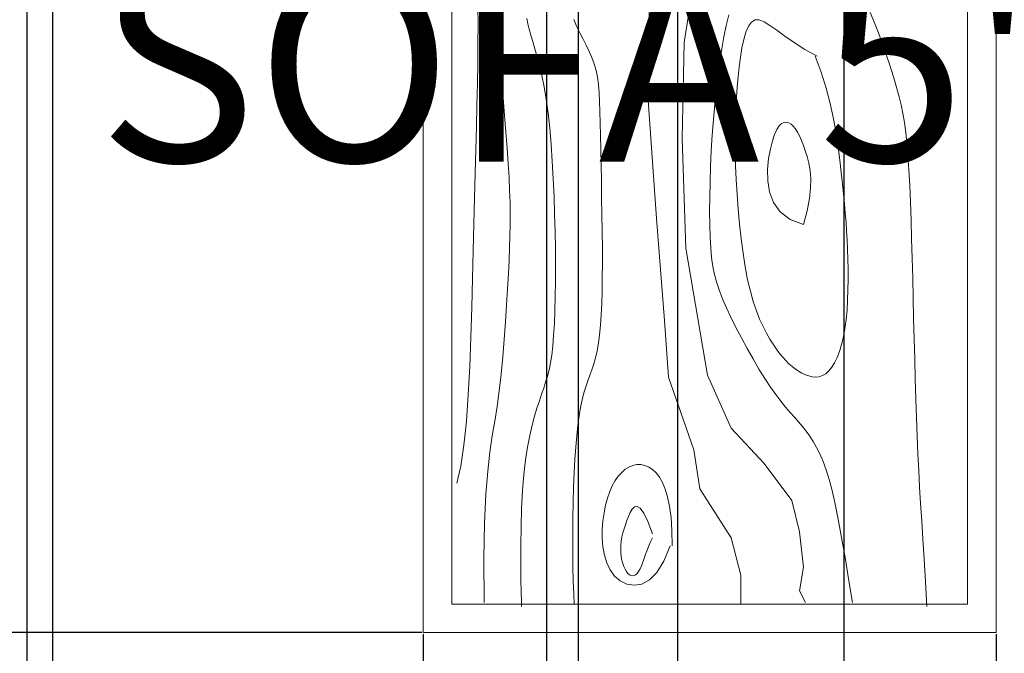
# Model space of a CAD drawing. Units: inches. Extents: x -26 to 385, y 12 to 697.
# Tile 6 of 13: x 223 to 264, y 165 to 191. Entities that reach past the tile are written whole.
import ezdxf

# ---------------------------------------------------------------- set-up
doc = ezdxf.new("R2010")
doc.units = ezdxf.units.IN
doc.header["$MEASUREMENT"] = 0
doc.layers.add('A-ANNO-DIMS', color=4, linetype='Continuous', lineweight=18)
doc.layers.add('Furniture', color=210, linetype='Continuous', lineweight=15)
doc.styles.get("Standard").update_dxf_attribs({"font": 'italic8.shx'})
doc.dimstyles.get("Standard").update_dxf_attribs({"dimtxt": 8, "dimasz": 0.18, "dimexe": 0.18, "dimexo": 0.0625, "dimgap": 0.09, "dimtad": 0, "dimtih": 1, "dimtoh": 1, "dimdec": 4, "dimzin": 0, "dimdsep": 46, "dimlunit": 3, "dimtxsty": 'Standard', "dimcen": 0.09, "dimclrd": 2, "dimclre": 3, "dimclrt": 6, "dimadec": 0, "dimazin": 0, "dimtfac": 1, "dimtdec": 4, "dimtofl": 0, "dimtmove": 0, "dimatfit": 3, "dimfxl": 1, "dimtolj": 1, "dimtzin": 0, "dimarcsym": 0})

# ---------------------------------------------------------------- blocks, each defined once
blk = doc.blocks.new('*D11')
at = {"layer": 'A-ANNO-DIMS', "color": 3, "lineweight": -2, "transparency": 16777216}
for p, q in [((285.56, 224.402), (274.992, 224.402)), ((285.56, 154.738), (274.992, 154.738))]:
    blk.add_line(p, q, dxfattribs=at)
at = {"layer": 'A-ANNO-DIMS', "color": 2, "lineweight": -2, "transparency": 16777216}
for p, q in [((275.172, 224.222), (275.172, 195.755)), ((275.172, 154.918), (275.172, 183.384))]:
    blk.add_line(p, q, dxfattribs=at)
at = {"layer": 'A-ANNO-DIMS', "color": 2, "transparency": 16777216}
for points in [[(275.142, 224.222), (275.202, 224.222), (275.172, 224.402)], [(275.142, 154.918), (275.202, 154.918), (275.172, 154.738)]]:
    blk.add_solid(points, dxfattribs=at)
at = {"layer": 'Defpoints', "color": 0, "transparency": 16777216}
for p in [(285.622, 224.402), (275.172, 154.738), (285.622, 154.738)]:
    blk.add_point(p, dxfattribs=at)
at = {"layer": 'A-ANNO-DIMS', "color": 6, "transparency": 16777216, "insert": (275.172, 189.57), "char_height": 8, "attachment_point": 5}
blk.add_mtext('\\A1;SOFA 5\'-9 1/2" TYP.', dxfattribs=at)
blk = doc.blocks.new('*D28')
at = {"layer": 'A-ANNO-DIMS', "color": 3, "lineweight": -2, "transparency": 16777216}
for p, q in [((141.692, 194.903), (355.559, 194.903)), ((141.692, 158.903), (355.559, 158.903))]:
    blk.add_line(p, q, dxfattribs=at)
at = {"layer": 'A-ANNO-DIMS', "color": 2, "lineweight": -2, "transparency": 16777216}
for p, q in [((355.379, 194.723), (355.379, 181.755)), ((355.379, 159.083), (355.379, 172.052))]:
    blk.add_line(p, q, dxfattribs=at)
at = {"layer": 'A-ANNO-DIMS', "color": 2, "transparency": 16777216}
for points in [[(355.349, 194.723), (355.409, 194.723), (355.379, 194.903)], [(355.349, 159.083), (355.409, 159.083), (355.379, 158.903)]]:
    blk.add_solid(points, dxfattribs=at)
at = {"layer": 'Defpoints', "color": 0, "transparency": 16777216}
for p in [(141.629, 194.903), (355.379, 194.903), (141.629, 158.903)]:
    blk.add_point(p, dxfattribs=at)
at = {"layer": 'A-ANNO-DIMS', "color": 6, "transparency": 16777216, "insert": (355.379, 176.903), "char_height": 8, "attachment_point": 5}
blk.add_mtext('\\A1;3\'-0"', dxfattribs=at)
blk = doc.blocks.new('*D31')
at = {"layer": 'A-ANNO-DIMS', "color": 3, "lineweight": -2, "transparency": 16777216}
for p, q in [((239.888, 166.079), (239.888, 23.949)), ((263.51, 166.079), (263.51, 23.949))]:
    blk.add_line(p, q, dxfattribs=at)
at = {"layer": 'A-ANNO-DIMS', "color": 2, "lineweight": -2, "transparency": 16777216}
for p, q in [((240.068, 24.129), (263.33, 24.129)), ((263.51, 24.129), (263.69, 24.129))]:
    blk.add_line(p, q, dxfattribs=at)
at = {"layer": 'A-ANNO-DIMS', "color": 2, "transparency": 16777216}
for points in [[(240.068, 24.159), (240.068, 24.099), (239.888, 24.129)], [(263.33, 24.159), (263.33, 24.099), (263.51, 24.129)]]:
    blk.add_solid(points, dxfattribs=at)
at = {"layer": 'Defpoints', "color": 0, "transparency": 16777216}
for p in [(239.888, 166.141), (263.51, 166.141), (263.51, 24.129)]:
    blk.add_point(p, dxfattribs=at)
at = {"layer": 'A-ANNO-DIMS', "color": 6, "transparency": 16777216, "insert": (296.732, 24.129), "char_height": 8, "attachment_point": 5}
blk.add_mtext('\\A1;1\'-11 1/2"', dxfattribs=at)
blk = doc.blocks.new('*D32')
at = {"layer": 'A-ANNO-DIMS', "color": 3, "lineweight": -2, "transparency": 16777216}
for p, q in [((239.825, 213.385), (-5.301, 213.385)), ((239.825, 166.141), (-5.301, 166.141))]:
    blk.add_line(p, q, dxfattribs=at)
at = {"layer": 'A-ANNO-DIMS', "color": 2, "lineweight": -2, "transparency": 16777216}
for p, q in [((-5.121, 213.205), (-5.121, 194.615)), ((-5.121, 166.321), (-5.121, 184.911))]:
    blk.add_line(p, q, dxfattribs=at)
at = {"layer": 'A-ANNO-DIMS', "color": 2, "transparency": 16777216}
for points in [[(-5.151, 213.205), (-5.091, 213.205), (-5.121, 213.385)], [(-5.151, 166.321), (-5.091, 166.321), (-5.121, 166.141)]]:
    blk.add_solid(points, dxfattribs=at)
at = {"layer": 'Defpoints', "color": 0, "transparency": 16777216}
for p in [(-5.121, 213.385), (239.888, 213.385), (239.888, 166.141)]:
    blk.add_point(p, dxfattribs=at)
at = {"layer": 'A-ANNO-DIMS', "color": 6, "transparency": 16777216, "insert": (-5.121, 189.763), "char_height": 8, "attachment_point": 5}
blk.add_mtext('\\A1;3\'-11"', dxfattribs=at)
blk = doc.blocks.new('*D35')
at = {"layer": 'A-ANNO-DIMS', "color": 3, "lineweight": -2, "transparency": 16777216}
for p, q in [((193.598, 147.942), (193.598, 684.809)), ((244.986, 147.942), (244.986, 684.809))]:
    blk.add_line(p, q, dxfattribs=at)
at = {"layer": 'A-ANNO-DIMS', "color": 2, "lineweight": -2, "transparency": 16777216}
for p, q in [((193.778, 684.629), (244.806, 684.629)), ((244.986, 684.629), (245.166, 684.629))]:
    blk.add_line(p, q, dxfattribs=at)
at = {"layer": 'A-ANNO-DIMS', "color": 2, "transparency": 16777216}
for points in [[(193.778, 684.659), (193.778, 684.599), (193.598, 684.629)], [(244.806, 684.659), (244.806, 684.599), (244.986, 684.629)]]:
    blk.add_solid(points, dxfattribs=at)
at = {"layer": 'Defpoints', "color": 0, "transparency": 16777216}
for p in [(244.986, 684.629), (193.598, 147.879), (244.986, 147.879)]:
    blk.add_point(p, dxfattribs=at)
at = {"layer": 'A-ANNO-DIMS', "color": 6, "transparency": 16777216, "insert": (278.398, 684.629), "char_height": 8, "attachment_point": 5}
blk.add_mtext('\\A1;4\'-3 1/2"', dxfattribs=at)
blk = doc.blocks.new('*D36')
at = {"layer": 'A-ANNO-DIMS', "color": 3, "lineweight": -2, "transparency": 16777216}
for p, q in [((146.129, 147.942), (146.129, 684.809)), ((193.598, 147.942), (193.598, 684.809))]:
    blk.add_line(p, q, dxfattribs=at)
at = {"layer": 'A-ANNO-DIMS', "color": 2, "lineweight": -2, "transparency": 16777216}
for p, q in [((146.309, 684.629), (193.418, 684.629)), ((193.598, 684.629), (193.778, 684.629))]:
    blk.add_line(p, q, dxfattribs=at)
at = {"layer": 'A-ANNO-DIMS', "color": 2, "transparency": 16777216}
for points in [[(146.309, 684.659), (146.309, 684.599), (146.129, 684.629)], [(193.418, 684.659), (193.418, 684.599), (193.598, 684.629)]]:
    blk.add_solid(points, dxfattribs=at)
at = {"layer": 'Defpoints', "color": 0, "transparency": 16777216}
for p in [(193.598, 684.629), (146.129, 147.879), (193.598, 147.879)]:
    blk.add_point(p, dxfattribs=at)
at = {"layer": 'A-ANNO-DIMS', "color": 6, "transparency": 16777216, "insert": (228.344, 684.629), "char_height": 8, "attachment_point": 5}
blk.add_mtext('\\A1;3\'-11 1/2"', dxfattribs=at)
blk = doc.blocks.new('*D37')
at = {"layer": 'A-ANNO-DIMS', "color": 3, "lineweight": -2, "transparency": 16777216}
for p, q in [((223.549, 597.317), (223.549, 23.949)), ((257.22, 597.317), (257.22, 23.949))]:
    blk.add_line(p, q, dxfattribs=at)
at = {"layer": 'A-ANNO-DIMS', "color": 2, "lineweight": -2, "transparency": 16777216}
for p, q in [((223.729, 24.129), (257.04, 24.129)), ((257.22, 24.129), (257.4, 24.129))]:
    blk.add_line(p, q, dxfattribs=at)
at = {"layer": 'A-ANNO-DIMS', "color": 2, "transparency": 16777216}
for points in [[(223.729, 24.159), (223.729, 24.099), (223.549, 24.129)], [(257.04, 24.159), (257.04, 24.099), (257.22, 24.129)]]:
    blk.add_solid(points, dxfattribs=at)
at = {"layer": 'Defpoints', "color": 0, "transparency": 16777216}
for p in [(223.549, 597.379), (257.22, 597.379), (257.22, 24.129)]:
    blk.add_point(p, dxfattribs=at)
at = {"layer": 'A-ANNO-DIMS', "color": 6, "transparency": 16777216, "insert": (290.633, 24.129), "char_height": 8, "attachment_point": 5}
blk.add_mtext('\\A1;2\'-9 1/2"', dxfattribs=at)
blk = doc.blocks.new('*D39')
at = {"layer": 'A-ANNO-DIMS', "color": 3, "lineweight": -2, "transparency": 16777216}
for p, q in [((183.359, 597.317), (183.359, 23.949)), ((213.359, 597.317), (213.359, 23.949))]:
    blk.add_line(p, q, dxfattribs=at)
at = {"layer": 'A-ANNO-DIMS', "color": 2, "lineweight": -2, "transparency": 16777216}
for p, q in [((183.539, 24.129), (213.179, 24.129)), ((213.359, 24.129), (213.539, 24.129))]:
    blk.add_line(p, q, dxfattribs=at)
at = {"layer": 'A-ANNO-DIMS', "color": 2, "transparency": 16777216}
for points in [[(183.539, 24.159), (183.539, 24.099), (183.359, 24.129)], [(213.179, 24.159), (213.179, 24.099), (213.359, 24.129)]]:
    blk.add_solid(points, dxfattribs=at)
at = {"layer": 'Defpoints', "color": 0, "transparency": 16777216}
for p in [(183.359, 597.379), (213.359, 597.379), (213.359, 24.129)]:
    blk.add_point(p, dxfattribs=at)
at = {"layer": 'A-ANNO-DIMS', "color": 6, "transparency": 16777216, "insert": (231.533, 24.129), "char_height": 8, "attachment_point": 5}
blk.add_mtext('\\A1;2\'-6"', dxfattribs=at)
blk = doc.blocks.new('*D42')
at = {"layer": 'A-ANNO-DIMS', "color": 3, "lineweight": -2, "transparency": 16777216}
for p, q in [((250.371, 518.992), (250.371, 23.949)), ((274.129, 518.992), (274.129, 23.949))]:
    blk.add_line(p, q, dxfattribs=at)
at = {"layer": 'A-ANNO-DIMS', "color": 2, "lineweight": -2, "transparency": 16777216}
for p, q in [((250.551, 24.129), (273.949, 24.129)), ((274.129, 24.129), (274.309, 24.129))]:
    blk.add_line(p, q, dxfattribs=at)
at = {"layer": 'A-ANNO-DIMS', "color": 2, "transparency": 16777216}
for points in [[(250.551, 24.159), (250.551, 24.099), (250.371, 24.129)], [(273.949, 24.159), (273.949, 24.099), (274.129, 24.129)]]:
    blk.add_solid(points, dxfattribs=at)
at = {"layer": 'Defpoints', "color": 0, "transparency": 16777216}
for p in [(250.371, 519.055), (274.129, 519.055), (274.129, 24.129)]:
    blk.add_point(p, dxfattribs=at)
at = {"layer": 'A-ANNO-DIMS', "color": 6, "transparency": 16777216, "insert": (292.304, 24.129), "char_height": 8, "attachment_point": 5}
blk.add_mtext('\\A1;2\'-0"', dxfattribs=at)
blk = doc.blocks.new('*D46')
at = {"layer": 'A-ANNO-DIMS', "color": 3, "lineweight": -2, "transparency": 16777216}
for p, q in [((224.595, 477.317), (224.595, 23.949)), ((284.629, 477.317), (284.629, 23.949))]:
    blk.add_line(p, q, dxfattribs=at)
at = {"layer": 'A-ANNO-DIMS', "color": 2, "lineweight": -2, "transparency": 16777216}
for p, q in [((224.775, 24.129), (236.617, 24.129)), ((284.449, 24.129), (272.607, 24.129))]:
    blk.add_line(p, q, dxfattribs=at)
at = {"layer": 'A-ANNO-DIMS', "color": 2, "transparency": 16777216}
for points in [[(224.775, 24.159), (224.775, 24.099), (224.595, 24.129)], [(284.449, 24.159), (284.449, 24.099), (284.629, 24.129)]]:
    blk.add_solid(points, dxfattribs=at)
at = {"layer": 'Defpoints', "color": 0, "transparency": 16777216}
for p in [(224.595, 477.379), (284.629, 477.379), (284.629, 24.129)]:
    blk.add_point(p, dxfattribs=at)
at = {"layer": 'A-ANNO-DIMS', "color": 6, "transparency": 16777216, "insert": (254.612, 24.129), "char_height": 8, "attachment_point": 5}
blk.add_mtext('\\A1;5\'-0"', dxfattribs=at)
blk = doc.blocks.new('*D50')
at = {"layer": 'A-ANNO-DIMS', "color": 3, "lineweight": -2, "transparency": 16777216}
for p, q in [((246.278, 401.871), (246.278, 23.949)), ((284.629, 398.317), (284.629, 23.949))]:
    blk.add_line(p, q, dxfattribs=at)
at = {"layer": 'A-ANNO-DIMS', "color": 2, "lineweight": -2, "transparency": 16777216}
for p, q in [((246.458, 24.129), (284.449, 24.129)), ((284.629, 24.129), (284.809, 24.129))]:
    blk.add_line(p, q, dxfattribs=at)
at = {"layer": 'A-ANNO-DIMS', "color": 2, "transparency": 16777216}
for points in [[(246.458, 24.159), (246.458, 24.099), (246.278, 24.129)], [(284.449, 24.159), (284.449, 24.099), (284.629, 24.129)]]:
    blk.add_solid(points, dxfattribs=at)
at = {"layer": 'Defpoints', "color": 0, "transparency": 16777216}
for p in [(246.278, 401.934), (284.629, 398.379), (284.629, 24.129)]:
    blk.add_point(p, dxfattribs=at)
at = {"layer": 'A-ANNO-DIMS', "color": 6, "transparency": 16777216, "insert": (318.042, 24.129), "char_height": 8, "attachment_point": 5}
blk.add_mtext('\\A1;3\'-2 1/2"', dxfattribs=at)

msp = doc.modelspace()

# ---------------------------------------------------------------- linework, layer by layer
at = {"layer": 'Furniture'}
for p, q in [((239.88756, 166.14113), (239.88756, 213.38513)), ((263.50956, 213.38513), (263.50956, 166.14113)), ((241.06866, 167.32223), (241.06866, 212.20403)), ((262.32846, 212.20403), (262.32846, 167.32223)), ((249.26214, 193.39853), (249.10065, 188.87448)), ((251.1193, 193.47931), (250.63482, 190.49021)), ((242.14138, 191.96625), (242.1424, 191.22463)), ((242.85064, 191.86926), (242.91269, 191.14289)), ((252.47852, 191.62122), (252.37572, 191.18868)), ((258.31298, 191.71684), (258.48609, 191.29892)), ((242.1424, 191.22463), (242.13822, 190.4475)), ((244.16233, 191.47311), (244.20257, 191.25411)), ((244.20257, 191.25411), (244.25591, 191.02879)), ((246.08743, 191.4343), (246.20915, 191.15418)), ((252.37572, 191.18868), (252.27939, 190.72079)), ((253.28986, 191.15523), (253.41478, 191.3285)), ((253.41478, 191.3285), (253.56186, 191.41926)), ((253.56186, 191.41926), (253.73411, 191.41965)), ((253.73411, 191.41965), (253.93688, 191.3391)), ((253.93688, 191.3391), (254.17608, 191.19133)), ((254.17608, 191.19133), (254.45763, 190.99008)), ((258.48609, 191.29892), (258.64973, 190.88226)), ((242.91269, 191.14289), (242.97743, 190.40942)), ((244.25591, 191.02879), (244.32351, 190.7868)), ((244.32351, 190.7868), (244.4031, 190.52177)), ((246.20915, 191.15418), (246.33876, 190.88541)), ((246.33876, 190.88541), (246.47137, 190.62486)), ((253.09673, 190.60971), (253.18466, 190.91158)), ((253.18466, 190.91158), (253.28986, 191.15523)), ((254.45763, 190.99008), (254.78743, 190.74906)), ((258.64973, 190.88226), (258.8036, 190.47001)), ((242.13822, 190.4475), (242.12931, 189.63661)), ((242.97743, 190.40942), (243.04343, 189.66972)), ((244.4031, 190.52177), (244.49152, 190.22834)), ((246.47137, 190.62486), (246.60208, 190.36935)), ((250.63482, 190.49021), (250.55408, 186.53167)), ((252.27939, 190.72079), (252.18968, 190.22008)), ((253.02362, 190.26176), (253.09673, 190.60971)), ((254.78743, 190.74906), (255.17141, 190.48201)), ((255.17141, 190.48201), (255.61547, 190.20265)), ((258.8036, 190.47001), (258.94738, 190.06535)), ((244.49152, 190.22834), (244.58562, 189.90114)), ((246.60208, 190.36935), (246.72601, 190.11573)), ((246.72601, 190.11573), (246.83827, 189.86085)), ((252.18968, 190.22008), (252.10675, 189.68908)), ((252.96289, 189.87989), (253.02362, 190.26176)), ((255.61547, 190.20265), (256.12553, 189.9247)), ((258.94738, 190.06535), (259.08074, 189.67141)), ((242.12931, 189.63661), (242.11614, 188.79369)), ((243.04343, 189.66972), (243.10927, 188.93002)), ((244.58562, 189.90114), (244.68224, 189.53481)), ((246.83827, 189.86085), (246.93397, 189.60156)), ((246.93397, 189.60156), (247.00954, 189.33403)), ((252.10675, 189.68908), (252.03076, 189.1303)), ((252.91209, 189.47625), (252.96289, 189.87989)), ((256.04479, 189.9247), (256.29361, 189.26091)), ((259.08074, 189.67141), (259.20339, 189.29135)), ((244.68224, 189.53481), (244.77823, 189.12399)), ((247.00954, 189.33403), (247.06666, 189.05183)), ((252.86879, 189.06298), (252.91209, 189.47625)), ((256.29361, 189.26091), (256.49867, 188.60572)), ((259.20339, 189.29135), (259.31499, 188.92834)), ((242.11614, 188.79369), (242.09919, 187.91978)), ((243.10927, 188.93002), (243.17354, 188.19789)), ((244.77823, 189.12399), (244.87044, 188.66331)), ((247.06666, 189.05183), (247.10832, 188.74786)), ((247.10832, 188.74786), (247.13752, 188.41501)), ((249.10065, 188.87448), (249.50438, 183.21942)), ((252.03076, 189.1303), (251.96187, 188.54628)), ((252.83104, 188.64937), (252.86879, 189.06298)), ((259.31499, 188.92834), (259.41542, 188.58315)), ((244.87044, 188.66331), (244.9557, 188.1474)), ((247.13752, 188.41501), (247.15726, 188.04618)), ((251.96187, 188.54628), (251.90023, 187.93954)), ((252.79898, 188.23324), (252.83104, 188.64937)), ((256.49867, 188.60572), (256.6654, 187.96393)), ((259.41542, 188.58315), (259.50529, 188.24712)), ((243.17354, 188.19789), (243.23481, 187.48091)), ((244.9557, 188.1474), (245.03148, 187.57343)), ((247.15726, 188.04618), (247.17053, 187.63428)), ((251.90023, 187.93954), (251.84601, 187.3126)), ((252.77322, 187.80953), (252.79898, 188.23324)), ((256.6654, 187.96393), (256.79926, 187.34038)), ((259.50529, 188.24712), (259.58538, 187.9092)), ((242.09919, 187.91978), (242.07892, 187.01313)), ((245.03148, 187.57343), (245.09764, 186.94864)), ((247.17053, 187.63428), (247.18034, 187.1722)), ((252.7544, 187.37319), (252.77322, 187.80953)), ((259.58538, 187.9092), (259.65648, 187.55833)), ((259.65648, 187.55833), (259.71938, 187.18348)), ((243.23481, 187.48091), (243.29166, 186.78665)), ((247.18034, 187.1722), (247.18967, 186.65285)), ((251.84601, 187.3126), (251.79938, 186.66915)), ((252.74315, 186.91919), (252.7544, 187.37319)), ((254.65677, 187.13974), (254.55688, 187.04247)), ((254.75738, 187.19132), (254.65677, 187.13974)), ((254.85719, 187.20235), (254.75738, 187.19132)), ((254.95472, 187.17796), (254.85719, 187.20235)), ((255.04878, 187.12268), (254.95472, 187.17796)), ((256.79926, 187.34038), (256.90567, 186.73985)), ((259.71938, 187.18348), (259.77486, 186.77361)), ((242.07892, 187.01313), (242.05582, 186.07129)), ((243.29166, 186.78665), (243.34268, 186.12269)), ((245.09764, 186.94864), (245.15465, 186.28284)), ((252.7401, 186.44247), (252.74315, 186.91919)), ((254.45919, 186.89441), (254.36521, 186.6904)), ((254.55688, 187.04247), (254.45919, 186.89441)), ((255.13945, 187.03869), (255.04878, 187.12268)), ((255.22712, 186.92755), (255.13945, 187.03869)), ((255.31219, 186.79086), (255.22712, 186.92755)), ((255.39505, 186.63018), (255.31219, 186.79086)), ((256.90567, 186.73985), (256.99008, 186.16718)), ((259.77486, 186.77361), (259.82373, 186.31766)), ((247.18967, 186.65285), (247.20087, 186.07261)), ((250.55408, 186.53167), (250.71557, 182.00762)), ((251.79938, 186.66915), (251.76064, 186.01749)), ((252.74588, 185.93797), (252.7401, 186.44247)), ((254.27644, 186.42533), (254.19436, 186.09407)), ((254.36521, 186.6904), (254.27644, 186.42533)), ((255.4761, 186.44709), (255.39505, 186.63018)), ((255.55573, 186.24318), (255.4761, 186.44709)), ((259.82373, 186.31766), (259.86675, 185.80459)), ((242.05582, 186.07129), (242.03035, 185.09182)), ((243.34268, 186.12269), (243.38644, 185.49659)), ((245.15465, 186.28284), (245.20299, 185.58579)), ((247.20087, 186.07261), (247.21364, 185.44189)), ((251.76064, 186.01749), (251.73009, 185.3671)), ((252.76113, 185.40066), (252.74588, 185.93797)), ((254.19436, 186.09407), (254.12362, 185.69644)), ((255.63433, 186.02002), (255.55573, 186.24318)), ((255.71091, 185.77771), (255.63433, 186.02002)), ((256.99008, 186.16718), (257.05793, 185.62717)), ((245.20299, 185.58579), (245.24312, 184.86729)), ((254.12362, 185.69644), (254.08134, 185.25202)), ((255.77889, 185.51047), (255.71091, 185.77771)), ((255.83032, 185.21105), (255.77889, 185.51047)), ((257.05793, 185.62717), (257.11467, 185.12463)), ((259.86675, 185.80459), (259.90471, 185.22651)), ((243.38644, 185.49659), (243.42153, 184.91594)), ((247.21364, 185.44189), (247.22705, 184.77456)), ((251.73009, 185.3671), (251.70807, 184.72743)), ((252.78639, 184.82818), (252.76113, 185.40066)), ((254.08134, 185.25202), (254.08779, 184.78535)), ((255.85722, 184.87218), (255.83032, 185.21105)), ((257.11467, 185.12463), (257.16486, 184.66228)), ((259.90471, 185.22651), (259.93825, 184.58816)), ((242.03035, 185.09182), (242.00299, 184.07227)), ((243.42153, 184.91594), (243.44687, 184.38464)), ((245.24312, 184.86729), (245.27553, 184.1371)), ((247.22705, 184.77456), (247.24013, 184.08451)), ((251.70807, 184.72743), (251.69487, 184.10796)), ((252.8219, 184.22904), (252.78639, 184.82818)), ((254.08779, 184.78535), (254.16324, 184.32098)), ((255.85164, 184.4866), (255.85722, 184.87218)), ((243.44687, 184.38464), (243.46275, 183.89201)), ((254.16324, 184.32098), (254.32795, 183.88342)), ((255.8056, 184.04706), (255.85164, 184.4866)), ((257.16486, 184.66228), (257.20961, 184.2344)), ((259.93825, 184.58816), (259.968, 183.89743)), ((242.00299, 184.07227), (241.97421, 183.01019)), ((243.46275, 183.89201), (243.46979, 183.42367)), ((245.27553, 184.1371), (245.30069, 183.40503)), ((247.24013, 184.08451), (247.25196, 183.38562)), ((251.69487, 184.10796), (251.69082, 183.51816)), ((252.86782, 183.61444), (252.8219, 184.22904)), ((254.32795, 183.88342), (254.60219, 183.49723)), ((255.71115, 183.5463), (255.8056, 184.04706)), ((257.20961, 184.2344), (257.24915, 183.83319)), ((259.968, 183.89743), (259.9946, 183.16219)), ((251.69082, 183.51816), (251.69624, 182.96749)), ((252.9243, 182.99557), (252.86782, 183.61444)), ((254.60219, 183.49723), (255.00622, 183.18693)), ((255.56031, 182.97706), (255.71115, 183.5463)), ((257.24915, 183.83319), (257.28373, 183.45084)), ((243.46979, 183.42367), (243.46863, 182.96528)), ((245.30069, 183.40503), (245.31906, 182.68084)), ((247.25196, 183.38562), (247.26158, 182.69178)), ((249.50438, 183.21942), (249.82736, 179.01851)), ((255.00622, 183.18693), (255.56031, 182.97706)), ((257.28373, 183.45084), (257.31358, 183.07953)), ((257.31358, 183.07953), (257.33893, 182.71145)), ((259.9946, 183.16219), (260.01868, 182.39036)), ((241.97421, 183.01019), (241.94448, 181.90315)), ((243.46863, 182.96528), (243.45991, 182.50246)), ((245.31906, 182.68084), (245.33102, 181.97359)), ((247.26158, 182.69178), (247.26805, 182.01688)), ((251.69624, 182.96749), (251.71143, 182.46541)), ((252.99151, 182.38365), (252.9243, 182.99557)), ((257.33893, 182.71145), (257.36002, 182.3388)), ((243.45991, 182.50246), (243.44424, 182.02087)), ((251.71143, 182.46541), (251.73703, 182.0179)), ((253.0696, 181.78987), (252.99151, 182.38365)), ((257.36002, 182.3388), (257.37709, 181.95376)), ((260.01868, 182.39036), (260.04086, 181.5898)), ((241.94448, 181.90315), (241.91428, 180.74869)), ((243.44424, 182.02087), (243.42227, 181.50615)), ((245.33102, 181.97359), (245.33651, 181.28938)), ((247.26805, 182.01688), (247.27041, 181.37479)), ((250.71557, 182.00762), (251.60377, 176.75649)), ((251.73703, 182.0179), (251.77493, 181.61694)), ((257.37709, 181.95376), (257.39013, 181.55085)), ((243.42227, 181.50615), (243.39462, 180.94393)), ((251.77493, 181.61694), (251.82735, 181.25101)), ((253.15873, 181.22545), (253.0696, 181.78987)), ((257.39013, 181.55085), (257.39812, 181.1339)), ((260.04086, 181.5898), (260.06178, 180.76842)), ((245.33651, 181.28938), (245.33538, 180.63356)), ((247.27041, 181.37479), (247.26779, 180.77683)), ((251.82735, 181.25101), (251.89647, 180.90858)), ((253.25906, 180.70157), (253.15873, 181.22545)), ((257.39812, 181.1339), (257.3998, 180.70906)), ((241.91428, 180.74869), (241.88321, 179.54985)), ((243.39462, 180.94393), (243.3617, 180.32466)), ((245.33538, 180.63356), (245.32747, 180.01152)), ((247.26779, 180.77683), (247.25948, 180.224)), ((251.89647, 180.90858), (251.98453, 180.57815)), ((253.3704, 180.22695), (253.25906, 180.70157)), ((257.3998, 180.70906), (257.39392, 180.28249)), ((260.06178, 180.76842), (260.08208, 179.9341)), ((243.3617, 180.32466), (243.32302, 179.65797)), ((247.25948, 180.224), (247.24487, 179.71472)), ((251.98453, 180.57815), (252.09371, 180.2482)), ((252.09371, 180.2482), (252.22624, 179.90719)), ((253.4912, 179.80029), (253.3704, 180.22695)), ((257.39392, 180.28249), (257.3792, 179.86033)), ((245.32747, 180.01152), (245.31262, 179.4286)), ((252.22624, 179.90719), (252.38431, 179.54363)), ((257.3792, 179.86033), (257.35438, 179.44875)), ((260.08208, 179.9341), (260.10233, 179.09429)), ((241.88321, 179.54985), (241.84741, 178.33151)), ((243.32302, 179.65797), (243.27788, 178.95831)), ((245.31262, 179.4286), (245.29067, 178.89018)), ((247.24487, 179.71472), (247.22331, 179.24741)), ((252.38431, 179.54363), (252.56891, 179.14956)), ((253.61958, 179.41782), (253.4912, 179.80029)), ((253.75363, 179.07574), (253.61958, 179.41782)), ((257.35438, 179.44875), (257.31822, 179.05389)), ((247.22331, 179.24741), (247.19419, 178.82049)), ((249.82736, 179.01851), (249.98886, 176.6757)), ((252.56891, 179.14956), (252.77606, 178.73134)), ((253.89146, 178.77026), (253.75363, 179.07574)), ((257.31822, 179.05389), (257.26943, 178.6819)), ((260.10233, 179.09429), (260.12297, 178.25472)), ((243.27788, 178.95831), (243.22556, 178.2401)), ((245.29067, 178.89018), (245.26147, 178.40162)), ((247.19419, 178.82049), (247.15687, 178.43239)), ((252.77606, 178.73134), (253.00055, 178.29893)), ((254.03119, 178.49761), (253.89146, 178.77026)), ((257.26943, 178.6819), (257.20716, 178.33809)), ((241.84741, 178.33151), (241.80215, 177.12407)), ((243.22556, 178.2401), (243.16535, 177.5178)), ((245.26147, 178.40162), (245.22486, 177.96829)), ((247.15687, 178.43239), (247.11071, 178.08153)), ((253.00055, 178.29893), (253.23719, 177.86226)), ((254.17092, 178.25399), (254.03119, 178.49761)), ((254.30875, 178.03561), (254.17092, 178.25399)), ((257.20716, 178.33809), (257.13212, 178.02425)), ((260.12297, 178.25472), (260.14441, 177.42068)), ((245.22486, 177.96829), (245.18072, 177.59276)), ((247.11071, 178.08153), (247.05509, 177.76632)), ((253.23719, 177.86226), (253.48077, 177.43126)), ((254.44328, 177.83906), (254.30875, 178.03561)), ((254.57496, 177.66239), (254.44328, 177.83906)), ((257.13212, 178.02425), (257.04541, 177.74134)), ((243.16535, 177.5178), (243.09655, 176.80582)), ((245.18072, 177.59276), (245.12918, 177.26646)), ((246.98985, 177.48404), (246.91673, 177.22732)), ((247.05509, 177.76632), (246.98985, 177.48404)), ((253.48077, 177.43126), (253.72608, 177.01589)), ((254.70476, 177.50403), (254.57496, 177.66239)), ((254.8336, 177.36239), (254.70476, 177.50403)), ((256.94813, 177.4903), (256.84139, 177.27208)), ((257.04541, 177.74134), (256.94813, 177.4903)), ((260.14441, 177.42068), (260.16703, 176.59744)), ((241.80215, 177.12407), (241.74269, 175.95788)), ((245.07038, 176.97802), (245.00449, 176.7161)), ((245.12918, 177.26646), (245.07038, 176.97802)), ((246.83793, 176.98765), (246.75566, 176.75649)), ((246.91673, 177.22732), (246.83793, 176.98765)), ((253.72608, 177.01589), (253.96792, 176.62608)), ((254.96245, 177.2359), (254.8336, 177.36239)), ((255.09224, 177.12298), (254.96245, 177.2359)), ((255.22393, 177.02204), (255.09224, 177.12298)), ((255.35845, 176.93153), (255.22393, 177.02204)), ((256.72629, 177.08763), (256.60394, 176.93789)), ((256.84139, 177.27208), (256.72629, 177.08763)), ((243.09655, 176.80582), (243.01845, 176.11863)), ((245.00449, 176.7161), (244.93165, 176.46932)), ((246.75566, 176.75649), (246.67213, 176.52533)), ((249.98886, 176.6757), (251.03855, 173.6866)), ((251.60377, 176.75649), (252.57272, 174.57525)), ((253.96792, 176.62608), (254.20109, 176.27177)), ((255.49642, 176.85069), (255.35845, 176.93153)), ((255.63706, 176.78216), (255.49642, 176.85069)), ((255.77929, 176.7294), (255.63706, 176.78216)), ((255.92199, 176.6959), (255.77929, 176.7294)), ((256.06405, 176.68512), (255.92199, 176.6959)), ((256.20439, 176.70053), (256.06405, 176.68512)), ((256.34188, 176.7456), (256.20439, 176.70053)), ((256.47543, 176.82381), (256.34188, 176.7456)), ((256.60394, 176.93789), (256.47543, 176.82381)), ((260.16703, 176.59744), (260.19122, 175.7903)), ((244.85204, 176.22633), (244.7658, 175.97576)), ((244.93165, 176.46932), (244.85204, 176.22633)), ((246.58954, 176.28566), (246.51011, 176.02894)), ((246.67213, 176.52533), (246.58954, 176.28566)), ((254.20109, 176.27177), (254.42144, 175.96006)), ((241.74269, 175.95788), (241.66431, 174.86333)), ((243.01845, 176.11863), (242.93033, 175.47064)), ((244.7658, 175.97576), (244.67309, 175.70626)), ((246.51011, 176.02894), (246.43604, 175.74666)), ((254.42144, 175.96006), (254.629, 175.6867)), ((260.19122, 175.7903), (260.21739, 175.00454)), ((242.93033, 175.47064), (242.8327, 174.86449)), ((244.57458, 175.40744), (244.47291, 175.0728)), ((244.67309, 175.70626), (244.57458, 175.40744)), ((246.36912, 175.43147), (246.30946, 175.08069)), ((246.43604, 175.74666), (246.36912, 175.43147)), ((254.629, 175.6867), (254.8249, 175.44458)), ((254.8249, 175.44458), (255.01023, 175.22659)), ((244.47291, 175.0728), (244.37124, 174.69683)), ((246.30946, 175.08069), (246.25673, 174.69284)), ((255.01023, 175.22659), (255.1861, 175.02565)), ((255.1861, 175.02565), (255.35361, 174.83465)), ((260.21739, 175.00454), (260.24592, 174.24544)), ((241.66431, 174.86333), (241.56228, 173.87079)), ((242.8327, 174.86449), (242.73088, 174.25558)), ((244.37124, 174.69683), (244.27273, 174.27399)), ((246.25673, 174.69284), (246.21063, 174.26641)), ((252.57272, 174.57525), (253.9454, 173.12109)), ((255.35361, 174.83465), (255.51387, 174.64649)), ((255.51387, 174.64649), (255.66797, 174.45407)), ((242.73088, 174.25558), (242.63144, 173.5875)), ((244.27273, 174.27399), (244.18052, 173.79876)), ((246.21063, 174.26641), (246.17083, 173.7999)), ((255.66797, 174.45407), (255.81689, 174.25049)), ((255.81689, 174.25049), (255.96099, 174.02963)), ((260.24592, 174.24544), (260.27721, 173.51829)), ((241.56228, 173.87079), (241.43185, 173.01063)), ((244.18052, 173.79876), (244.09778, 173.26563)), ((246.17083, 173.7999), (246.13703, 173.29182)), ((255.96099, 174.02963), (256.10052, 173.78557)), ((256.10052, 173.78557), (256.23572, 173.5124)), ((242.63144, 173.5875), (242.5409, 172.80384)), ((251.03855, 173.6866), (251.28079, 172.07087)), ((256.23572, 173.5124), (256.36681, 173.20421)), ((260.27721, 173.51829), (260.31161, 172.82397)), ((241.43185, 173.01063), (241.26831, 172.31323)), ((244.09778, 173.26563), (244.02765, 172.66906)), ((246.13703, 173.29182), (246.10891, 172.74066)), ((248.36728, 172.97454), (248.21245, 172.87873)), ((248.52755, 173.03925), (248.36728, 172.97454)), ((248.69113, 173.0721), (248.52755, 173.03925)), ((248.85589, 173.07228), (248.69113, 173.0721)), ((249.01971, 173.03902), (248.85589, 173.07228)), ((249.18045, 172.97151), (249.01971, 173.03902)), ((249.33599, 172.86898), (249.18045, 172.97151)), ((253.9454, 173.12109), (255.07584, 171.58615)), ((256.36681, 173.20421), (256.49404, 172.85507)), ((242.5409, 172.80384), (242.46582, 171.84819)), ((244.02765, 172.66906), (243.9733, 172.00355)), ((246.10891, 172.74066), (246.08614, 172.14492)), ((247.92626, 172.59703), (247.79729, 172.41271)), ((248.06502, 172.75264), (247.92626, 172.59703)), ((248.21245, 172.87873), (248.06502, 172.75264)), ((249.48419, 172.73062), (249.33599, 172.86898)), ((249.62294, 172.55467), (249.48419, 172.73062)), ((249.75009, 172.33532), (249.62294, 172.55467)), ((256.49404, 172.85507), (256.61764, 172.45906)), ((260.31161, 172.82397), (260.34923, 172.14566)), ((246.08614, 172.14492), (246.06853, 171.50645)), ((247.67919, 172.20046), (247.57308, 171.96107)), ((247.79729, 172.41271), (247.67919, 172.20046)), ((249.86352, 172.06579), (249.75009, 172.33532)), ((256.61764, 172.45906), (256.73786, 172.01028)), ((260.34923, 172.14566), (260.39017, 171.46214)), ((242.46582, 171.84819), (242.41274, 170.66415)), ((243.9733, 172.00355), (243.93679, 171.27076)), ((247.57308, 171.96107), (247.48006, 171.69534)), ((249.9611, 171.73931), (249.86352, 172.06579)), ((250.0407, 171.34907), (249.9611, 171.73931)), ((251.28079, 172.07087), (252.57272, 170.0512)), ((256.73786, 172.01028), (256.85486, 171.50587)), ((246.06853, 171.50645), (246.05628, 170.84045)), ((247.40123, 171.40404), (247.3377, 171.08796)), ((247.48006, 171.69534), (247.40123, 171.40404)), ((248.59589, 171.32944), (248.50263, 171.23807)), ((248.70365, 171.348), (248.59589, 171.32944)), ((248.82908, 171.26967), (248.70365, 171.348)), ((250.1002, 170.88831), (250.0407, 171.34907)), ((255.07584, 171.58615), (255.39882, 170.29356)), ((256.85486, 171.50587), (256.96863, 170.95532)), ((260.39017, 171.46214), (260.4345, 170.75219)), ((243.93679, 171.27076), (243.91589, 170.50121)), ((247.3377, 171.08796), (247.29109, 170.7493)), ((248.34702, 170.93312), (248.27905, 170.76373)), ((248.42073, 171.09794), (248.34702, 170.93312)), ((248.50263, 171.23807), (248.42073, 171.09794)), ((248.97533, 171.0704), (248.82908, 171.26967)), ((249.14555, 170.72612), (248.97533, 171.0704)), ((250.13745, 170.35023), (250.1002, 170.88831)), ((256.96863, 170.95532), (257.07909, 170.37115)), ((242.41274, 170.66415), (242.3882, 169.1953)), ((243.91589, 170.50121), (243.9073, 169.73261)), ((246.05628, 170.84045), (246.04971, 170.16545)), ((247.29109, 170.7493), (247.26505, 170.39581)), ((248.21707, 170.59409), (248.16203, 170.42462)), ((248.27905, 170.76373), (248.21707, 170.59409)), ((249.34289, 170.21278), (249.14555, 170.72612)), ((260.4345, 170.75219), (260.4823, 169.9946)), ((246.04971, 170.16545), (246.04913, 169.5)), ((247.26505, 170.39581), (247.26378, 170.03663)), ((248.07656, 170.08772), (248.04801, 169.92108)), ((248.11488, 170.25569), (248.07656, 170.08772)), ((248.16203, 170.42462), (248.11488, 170.25569)), ((250.15035, 169.72806), (250.13745, 170.35023)), ((255.39882, 170.29356), (255.56031, 168.8394)), ((257.07909, 170.37115), (257.18616, 169.76593)), ((243.9073, 169.73261), (243.90769, 169.00266)), ((247.26378, 170.03663), (247.29144, 169.68093)), ((247.29144, 169.68093), (247.35222, 169.33785)), ((248.03019, 169.75618), (248.02404, 169.59341)), ((248.04801, 169.92108), (248.03019, 169.75618)), ((249.11331, 169.55063), (249.1815, 169.72448)), ((249.1815, 169.72448), (249.25743, 169.89297)), ((249.25743, 169.89297), (249.34289, 170.0512)), ((249.80845, 169.09273), (250.0696, 169.72806)), ((252.57272, 170.0512), (252.97645, 168.51626)), ((257.18616, 169.76593), (257.28976, 169.15218)), ((260.4823, 169.9946), (260.53364, 169.16813)), ((246.04913, 169.5), (246.05486, 168.86264)), ((247.35222, 169.33785), (247.45031, 169.01655)), ((248.02404, 169.59341), (248.03014, 169.4335)), ((248.03014, 169.4335), (248.04759, 169.27847)), ((248.04759, 169.27847), (248.07514, 169.1307)), ((248.99285, 169.20639), (249.05103, 169.3763)), ((249.05103, 169.3763), (249.11331, 169.55063)), ((242.3882, 169.1953), (242.39875, 167.38525)), ((243.90769, 169.00266), (243.91376, 168.34908)), ((246.05486, 168.86264), (246.06722, 168.2719)), ((247.45031, 169.01655), (247.58986, 168.72617)), ((248.07514, 169.1307), (248.11152, 168.99256)), ((248.11152, 168.99256), (248.15546, 168.86641)), ((248.15546, 168.86641), (248.20572, 168.75462)), ((248.82477, 168.77208), (248.88153, 168.89939)), ((248.88153, 168.89939), (248.93695, 169.04579)), ((248.93695, 169.04579), (248.99285, 169.20639)), ((249.5171, 168.62923), (249.80845, 169.09273)), ((257.28976, 169.15218), (257.38981, 168.54245)), ((260.53364, 169.16813), (260.58862, 168.25156)), ((247.58986, 168.72617), (247.77508, 168.47586)), ((247.77508, 168.47586), (248.00752, 168.27619)), ((248.20572, 168.75462), (248.26102, 168.65955)), ((248.26102, 168.65955), (248.32011, 168.58358)), ((248.32011, 168.58358), (248.38181, 168.52872)), ((248.38181, 168.52872), (248.44533, 168.49564)), ((248.44533, 168.49564), (248.50995, 168.48465)), ((248.50995, 168.48465), (248.57496, 168.49606)), ((248.57496, 168.49606), (248.63966, 168.5302)), ((248.63966, 168.5302), (248.70334, 168.58737)), ((248.70334, 168.58737), (248.76528, 168.66789)), ((248.76528, 168.66789), (248.82477, 168.77208)), ((249.20699, 168.32005), (249.5171, 168.62923)), ((252.97645, 168.51626), (252.97645, 167.30446)), ((255.56031, 168.8394), (255.39882, 167.86996)), ((257.38981, 168.54245), (257.48624, 167.94929)), ((243.91376, 168.34908), (243.9222, 167.80959)), ((246.06722, 168.2719), (246.08651, 167.74633)), ((248.00752, 168.27619), (248.27837, 168.14325)), ((248.27837, 168.14325), (248.57619, 168.09457)), ((248.57619, 168.09457), (248.88954, 168.14767)), ((248.88954, 168.14767), (249.20699, 168.32005)), ((260.58862, 168.25156), (260.6473, 167.22367)), ((243.9222, 167.80959), (243.92969, 167.42188)), ((246.08651, 167.74633), (246.11306, 167.30446)), ((255.39882, 167.86996), (255.64106, 167.38525)), ((257.48624, 167.94929), (257.57896, 167.38525)), ((262.32846, 167.32223), (241.06866, 167.32223)), ((243.92969, 167.42188), (243.93292, 167.22367)), ((263.50956, 166.14113), (239.88756, 166.14113))]:
    msp.add_line(p, q, dxfattribs=at)

# ---------------------------------------------------------------- dimensions: what is measured, and where the dimension line sits
at = {"layer": 'A-ANNO-DIMS'}
for base, p1, p2, picture, middle in [((193.59818, 684.62909), (146.12932, 147.87909), (193.59818, 147.87909), '*D36', (228.34437, 684.62909)), ((244.98557, 684.62909), (193.59818, 147.87909), (244.98557, 147.87909), '*D35', (278.39843, 684.62909)), ((213.35855, 24.12909), (183.35855, 597.37909), (213.35855, 597.37909), '*D39', (231.53331, 24.12909)), ((257.21981, 24.12909), (223.54856, 597.37909), (257.21981, 597.37909), '*D37', (290.63267, 24.12909)), ((274.12932, 24.12909), (250.37102, 519.05498), (274.12932, 519.05498), '*D42', (292.30408, 24.12909)), ((284.62932, 24.12909), (224.59493, 477.37909), (284.62932, 477.37909), '*D46', (254.61213, 24.12909)), ((284.62932, 24.12909), (246.27828, 401.934), (284.62932, 398.37909), '*D50', (318.04218, 24.12909)), ((263.50956, 24.12909), (239.88756, 166.14113), (263.50956, 166.14113), '*D31', (296.73194, 24.12909))]:
    dim = msp.add_linear_dim(base=base, p1=p1, p2=p2, dimstyle='Standard', override={"dimdec": 1, "dimlfac": 1, "dimrnd": 0, "dimzin": 1, "dimdsep": 46, "dimlunit": 4, "dimfrac": 2}, dxfattribs=at)
    dim.commit()
    dim.dimension.update_dxf_attribs({"geometry": picture, "text_midpoint": middle})
dim = msp.add_linear_dim(base=(275.17245, 154.73754), p1=(285.62207, 224.40165), p2=(285.62207, 154.73754), angle=270, text='SOFA <> TYP.', dimstyle='Standard', override={"dimdec": 1, "dimlfac": 1, "dimrnd": 0, "dimzin": 1, "dimdsep": 46, "dimlunit": 4, "dimfrac": 2}, dxfattribs=at)
dim.commit()
dim.dimension.update_dxf_attribs({"geometry": '*D11', "text_midpoint": (275.17245, 189.56959)})
for base, p1, p2, picture, middle in [((-5.12068, 213.38513), (239.88756, 166.14113), (239.88756, 213.38513), '*D32', (-5.12068, 189.76313)), ((355.37932, 194.90341), (141.62932, 158.90341), (141.62932, 194.90341), '*D28', (355.37932, 176.90341))]:
    dim = msp.add_linear_dim(base=base, p1=p1, p2=p2, angle=90, dimstyle='Standard', override={"dimdec": 1, "dimlfac": 1, "dimrnd": 0, "dimzin": 1, "dimdsep": 46, "dimlunit": 4, "dimfrac": 2}, dxfattribs=at)
    dim.commit()
    dim.dimension.update_dxf_attribs({"geometry": picture, "text_midpoint": middle})

doc.saveas('drawing.dxf')
